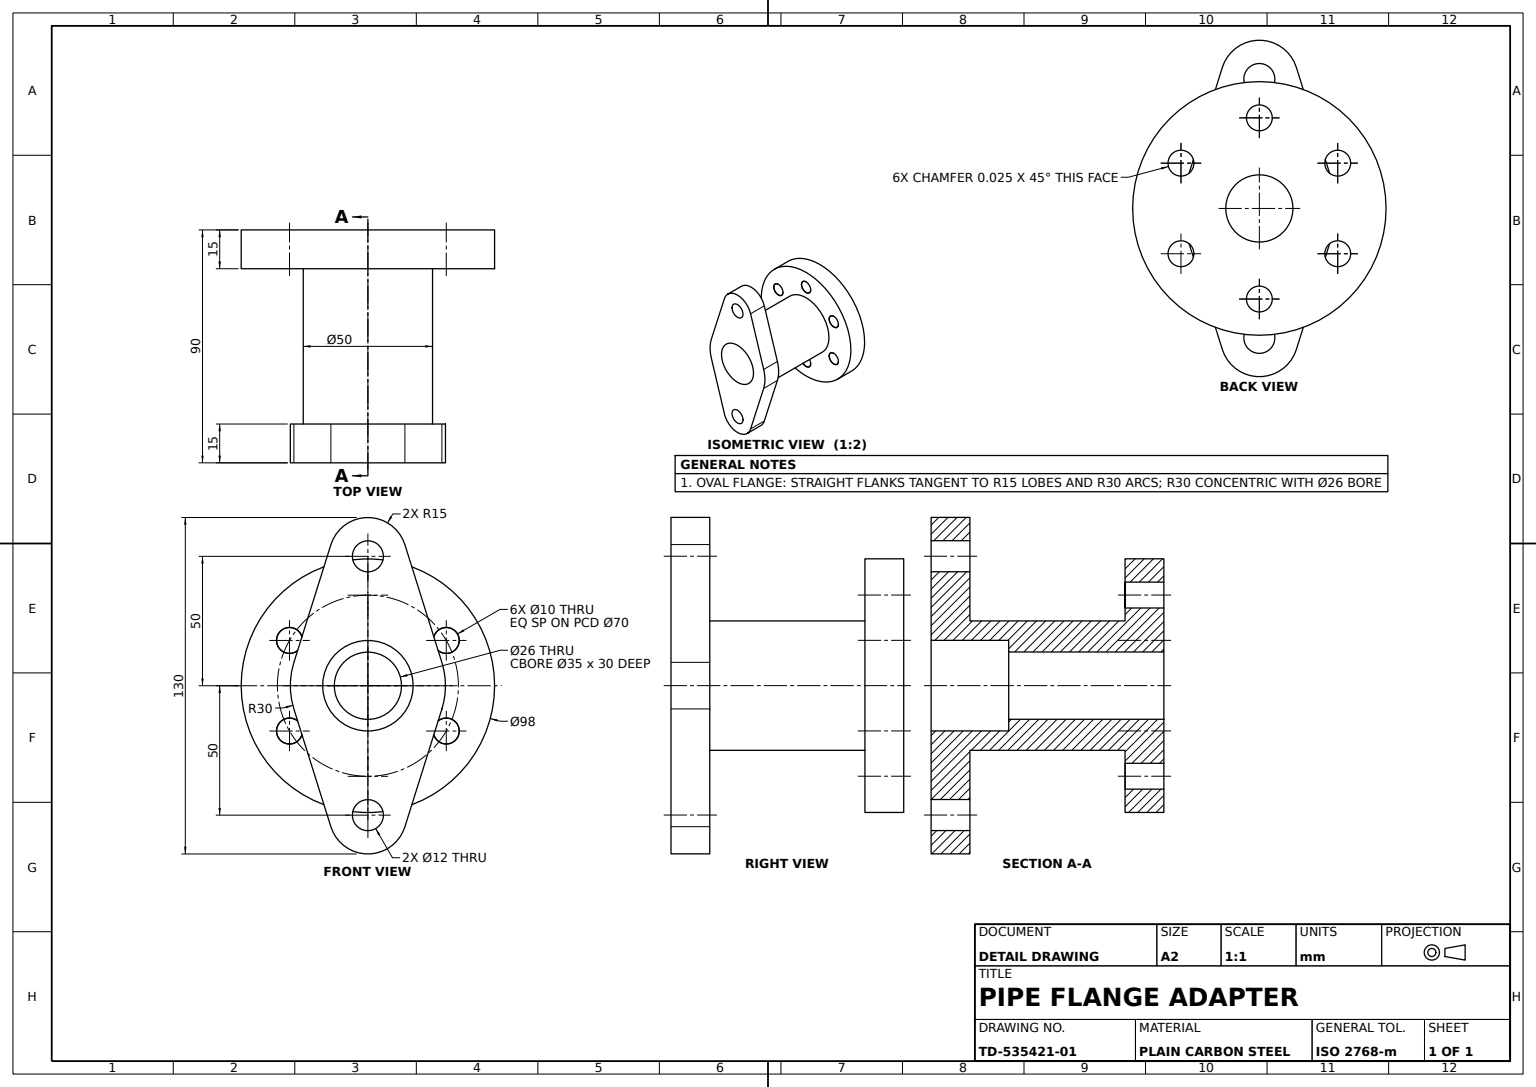
from build123d import *

# Parameters (mm, degrees)
FLANGE_AND_TUBE_PROFILE_SKETCH_R   = 49
FLANGE_AND_TUBE_PROFILE_SKETCH_R_2 = 25
ROUND_FLANGE_98_DEPTH              = 15
SKETCH1_3_R                        = 25
SKETCH1_3_R_2                      = 13
TUBE_BODY_50_DEPTH                 = 90
OVAL_START                         = -15
OVAL_FLANGE_PROFILE_SKETCH_R       = 6
OVAL_FLANGE_PROFILE_SKETCH_R_2     = 25
OVAL_MOUNTING_FLANGE_DEPTH         = 15
SKETCH2_3_R                        = 17.5
OVAL_FLANGE_BORE_CUT_DEPTH         = 30
FLANGE_HOLES_6X_10_D               = 10
FLANGE_HOLES_6X_10_DEPTH           = 15
FLANGE_HOLES_6X_10_CSINK_D         = 10.05
FLANGE_HOLES_6X_10_CSINK_ANGLE     = 90


with BuildPart() as part:
    # Flange and Tube Profile Sketch → Round Flange _98 (new body)
    with BuildSketch(Plane.XY):
        Circle(FLANGE_AND_TUBE_PROFILE_SKETCH_R)
        Circle(FLANGE_AND_TUBE_PROFILE_SKETCH_R_2, mode=Mode.SUBTRACT)
    extrude(amount=ROUND_FLANGE_98_DEPTH)

    # Sketch1_3 → Tube Body _50 (add)
    with BuildSketch(Plane.XY):
        with Locations(Location((0, 0, 0), (0, 0, 180))):
            Circle(SKETCH1_3_R)
        with Locations(Location((0, 0, 0), (0, 0, 180))):
            Circle(SKETCH1_3_R_2, mode=Mode.SUBTRACT)
    extrude(amount=TUBE_BODY_50_DEPTH)

    # Oval Flange Profile Sketch → Oval Mounting Flange (add)
    with BuildSketch(Plane.XY.offset(90).offset(OVAL_START)):
        with BuildLine():
            Line((14.309088021, -54.5), (28.618176043, -9))
            ThreePointArc((28.618176043, -9), (30, 0), (28.618176043, 9))
            Line((28.618176043, 9), (14.309088021, 54.5))
            ThreePointArc((14.309088021, 54.5), (0, 65), (-14.309088021, 54.5))
            Line((-14.309088021, 54.5), (-28.618176043, 9))
            ThreePointArc((-28.618176043, 9), (-30, 0), (-28.618176043, -9))
            Line((-28.618176043, -9), (-14.309088021, -54.5))
            ThreePointArc((-14.309088021, -54.5), (0, -65), (14.309088021, -54.5))
        make_face()
        with Locations((0, -50)):
            Circle(OVAL_FLANGE_PROFILE_SKETCH_R, mode=Mode.SUBTRACT)
        with Locations((0, 50)):
            Circle(OVAL_FLANGE_PROFILE_SKETCH_R, mode=Mode.SUBTRACT)
        with Locations(Location((0, 0, 0), (0, 0, 180))):
            Circle(OVAL_FLANGE_PROFILE_SKETCH_R_2, mode=Mode.SUBTRACT)
    extrude(amount=OVAL_MOUNTING_FLANGE_DEPTH)

    # Sketch2_3 → Oval Flange Bore Cut (cut)
    with BuildSketch(Plane.XY.offset(90)):
        Circle(SKETCH2_3_R)
    extrude(amount=-OVAL_FLANGE_BORE_CUT_DEPTH, mode=Mode.SUBTRACT)

    # Flange Holes 6x_10
    with Locations(Plane.XY.offset(15)):
        with Locations((-30.310889132, 17.5), (0, 35), (30.310889132, 17.5), (30.310889132, -17.5), (0, -35), (-30.310889132, -17.5)):
            CounterSinkHole(FLANGE_HOLES_6X_10_D / 2, FLANGE_HOLES_6X_10_CSINK_D / 2, depth=FLANGE_HOLES_6X_10_DEPTH, counter_sink_angle=FLANGE_HOLES_6X_10_CSINK_ANGLE)


solid = part.part
